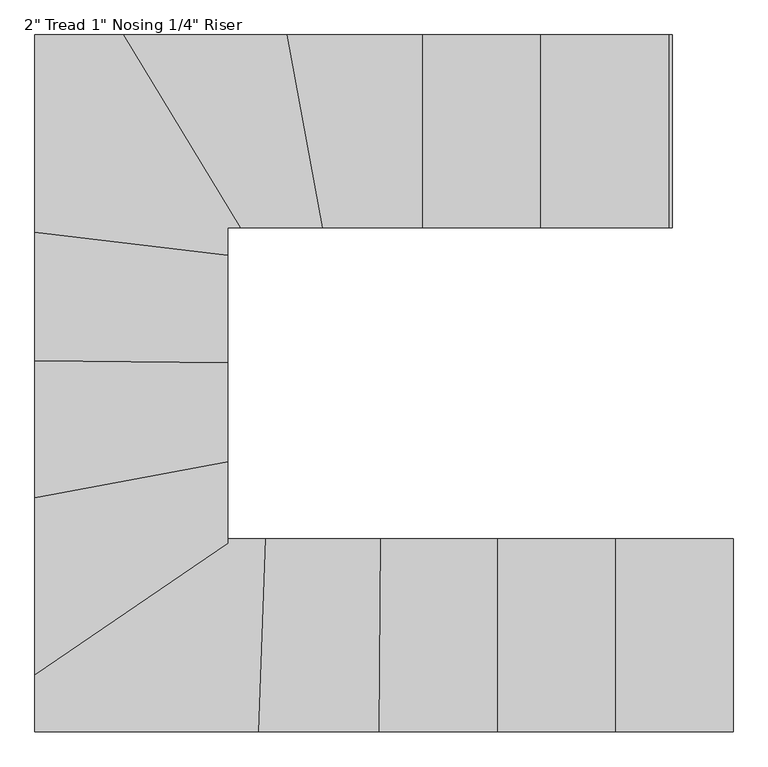
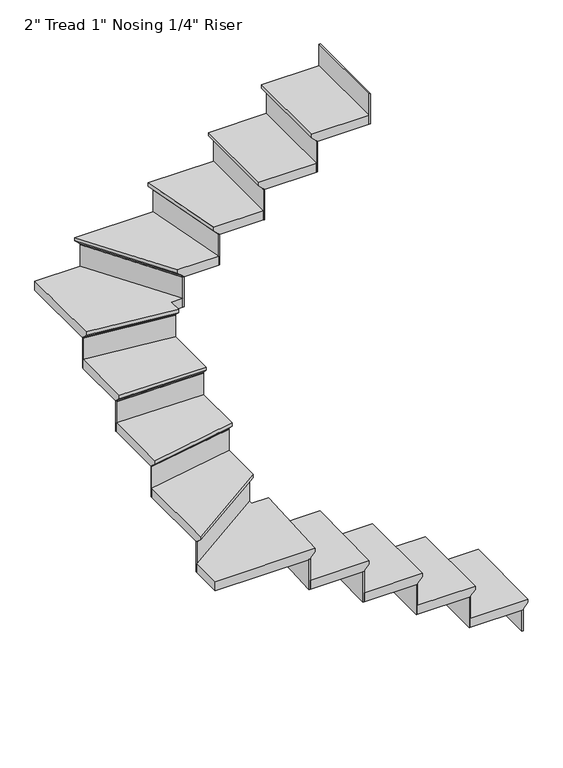
"""IFC4 building model written with IfcOpenShell, lengths in millimetres: stair flight geometry."""

from ifc_helpers import new_model, si_unit, origin, place, context, project, spatial, faceted_brep, source, transform, mapped, element, save


def stair_flight_132ddc74(model_context):
    return source(origin(), model_context, "Body", "Brep", [
        faceted_brep([(-10847.2047602, 4039.299435, 488.95), (-10847.2047602, 4039.299435, 508.0), (-10847.2047602, 3582.099435, 508.0), (-10847.2047602, 3582.099435, 488.95), (-10872.6047602, 4039.299435, 463.55), (-10872.6047602, 3582.099435, 463.55), (-11152.0047602, 4039.299435, 508.0), (-11152.0047602, 3582.099435, 508.0), (-10872.6047602, 3582.099435, 457.2), (-11152.0047602, 3582.099435, 457.2), (-11152.0047602, 4039.299435, 457.2), (-10872.6047602, 4039.299435, 457.2)], [[[0, 1, 2, 3]], [[4, 0, 3, 5]], [[2, 1, 6, 7]], [[8, 9, 10, 11]], [[2, 7, 9, 8, 5, 3]], [[8, 11, 4, 5]], [[6, 1, 0, 4, 11, 10]], [[7, 6, 10, 9]]]),
        faceted_brep([(-10872.6047602, 4039.299435, 457.2), (-10872.6047602, 4039.299435, 338.6666667), (-10878.9547602, 4039.299435, 338.6666667), (-10878.9547602, 4039.299435, 457.2), (-10872.6047602, 3582.099435, 457.2), (-10878.9547602, 3582.099435, 457.2), (-10878.9547602, 3582.099435, 338.6666667), (-10872.6047602, 3582.099435, 338.6666667)], [[[0, 1, 2, 3]], [[4, 5, 6, 7]], [[1, 0, 4, 7]], [[2, 1, 7, 6]], [[3, 2, 6, 5]], [[0, 3, 5, 4]]]),
        faceted_brep([(-11152.0047602, 4039.299435, 626.5333333), (-11152.0047602, 4039.299435, 457.2), (-11158.3547602, 4039.299435, 457.2), (-11158.3547602, 4039.299435, 626.5333333), (-11152.0047602, 3582.099435, 626.5333333), (-11158.3547602, 3582.099435, 626.5333333), (-11158.3547602, 3582.099435, 457.2), (-11152.0047602, 3582.099435, 457.2)], [[[0, 1, 2, 3]], [[4, 5, 6, 7]], [[1, 0, 4, 7]], [[2, 1, 7, 6]], [[3, 2, 6, 5]], [[0, 3, 5, 4]]]),
        faceted_brep([(-11126.6047602, 3582.099435, 677.3333333), (-11126.6047602, 4039.299435, 677.3333333), (-11431.4047602, 4039.299435, 677.3333333), (-11431.4047602, 3582.099435, 677.3333333), (-11152.0047602, 3582.099435, 626.5333333), (-11431.4047602, 3582.099435, 626.5333333), (-11431.4047602, 4039.299435, 626.5333333), (-11152.0047602, 4039.299435, 626.5333333), (-11152.0047602, 3582.099435, 632.8833333), (-11126.6047602, 3582.099435, 658.2833333), (-11152.0047602, 4039.299435, 632.8833333), (-11126.6047602, 4039.299435, 658.2833333)], [[[0, 1, 2, 3]], [[4, 5, 6, 7]], [[0, 3, 5, 4, 8, 9]], [[4, 7, 10, 8]], [[2, 1, 11, 10, 7, 6]], [[3, 2, 6, 5]], [[11, 1, 0, 9]], [[10, 11, 9, 8]]]),
        faceted_brep([(-11431.4047602, 4039.299435, 795.8666667), (-11431.4047602, 4039.299435, 626.5333333), (-11437.7547602, 4039.299435, 626.5333333), (-11437.7547602, 4039.299435, 795.8666667), (-11431.4047602, 3582.099435, 795.8666667), (-11437.7547602, 3582.099435, 795.8666667), (-11437.7547602, 3582.099435, 626.5333333), (-11431.4047602, 3582.099435, 626.5333333)], [[[0, 1, 2, 3]], [[4, 5, 6, 7]], [[1, 0, 4, 7]], [[2, 1, 7, 6]], [[3, 2, 6, 5]], [[0, 3, 5, 4]]]),
        faceted_brep([(-11406.0047602, 3582.099435, 846.6666667), (-11406.0047602, 4039.299435, 846.6666667), (-11708.6929844, 4039.299435, 846.6666667), (-11712.9187058, 3582.099435, 846.6666667), (-11431.4047602, 3582.099435, 795.8666667), (-11712.9187058, 3582.099435, 795.8666667), (-11708.6929844, 4039.299435, 795.8666667), (-11431.4047602, 4039.299435, 795.8666667), (-11431.4047602, 3582.099435, 802.2166667), (-11406.0047602, 3582.099435, 827.6166667), (-11431.4047602, 4039.299435, 802.2166667), (-11406.0047602, 4039.299435, 827.6166667)], [[[0, 1, 2, 3]], [[4, 5, 6, 7]], [[0, 3, 5, 4, 8, 9]], [[4, 7, 10, 8]], [[2, 1, 11, 10, 7, 6]], [[3, 2, 6, 5]], [[11, 1, 0, 9]], [[10, 11, 9, 8]]]),
        faceted_brep([(-11708.6929844, 4039.299435, 965.2), (-11708.6929844, 4039.299435, 795.8666667), (-11715.0432556, 4039.299435, 795.8666667), (-11715.0432556, 4039.299435, 965.2), (-11712.9187058, 3582.099435, 965.2), (-11719.268977, 3582.099435, 965.2), (-11719.268977, 3582.099435, 795.8666667), (-11712.9187058, 3582.099435, 795.8666667)], [[[0, 1, 2, 3]], [[4, 5, 6, 7]], [[1, 0, 4, 7]], [[2, 1, 7, 6]], [[3, 2, 6, 5]], [[0, 3, 5, 4]]]),
        faceted_brep([(-11687.5176209, 3582.099435, 1016.0), (-11683.2918995, 4039.299435, 1016.0), (-11981.9484639, 4039.299435, 1016.0), (-11998.4943115, 3582.099435, 1016.0), (-11712.9187058, 3582.099435, 965.2), (-11998.4943115, 3582.099435, 965.2), (-11981.9484639, 4039.299435, 965.2), (-11708.6929844, 4039.299435, 965.2), (-11712.9187058, 3582.099435, 971.55), (-11687.5176209, 3582.099435, 996.95), (-11708.6929844, 4039.299435, 971.55), (-11683.2918995, 4039.299435, 996.95)], [[[0, 1, 2, 3]], [[4, 5, 6, 7]], [[0, 3, 5, 4, 8, 9]], [[4, 7, 10, 8]], [[2, 1, 11, 10, 7, 6]], [[3, 2, 6, 5]], [[11, 1, 0, 9]], [[10, 11, 9, 8]]]),
        faceted_brep([(-11981.9484639, 4039.299435, 1134.5333333), (-11981.9484639, 4039.299435, 965.2), (-11988.3026208, 4039.299435, 965.2), (-11988.3026208, 4039.299435, 1134.5333333), (-11998.4943115, 3582.099435, 1134.5333333), (-12004.8484684, 3582.099435, 1134.5333333), (-12004.8484684, 3582.099435, 965.2), (-11998.4943115, 3582.099435, 965.2)], [[[0, 1, 2, 3]], [[4, 5, 6, 7]], [[1, 0, 4, 7]], [[2, 1, 7, 6]], [[3, 2, 6, 5]], [[0, 3, 5, 4]]]),
        faceted_brep([(-12501.9364521, 3747.8081502, 1185.3333333), (-12501.9364521, 3582.099435, 1185.3333333), (-11973.077684, 3582.099435, 1185.3333333), (-11956.5318364, 4039.299435, 1185.3333333), (-12044.7364521, 4039.299435, 1185.3333333), (-12044.7364521, 4058.9952275, 1185.3333333), (-12501.9364521, 3582.099435, 1134.5333333), (-12501.9364521, 3747.8081502, 1134.5333333), (-12044.7364521, 4058.9952275, 1134.5333333), (-12044.7364521, 4039.299435, 1134.5333333), (-11981.9484639, 4039.299435, 1134.5333333), (-11998.4943115, 3582.099435, 1134.5333333), (-11981.9484639, 4039.299435, 1140.8833333), (-11998.4943115, 3582.099435, 1140.8833333), (-11956.5318364, 4039.299435, 1166.2833333), (-11973.077684, 3582.099435, 1166.2833333)], [[[0, 1, 2, 3, 4, 5]], [[6, 7, 8, 9, 10, 11]], [[1, 0, 7, 6]], [[11, 10, 12, 13]], [[4, 3, 14, 12, 10, 9]], [[0, 5, 8, 7]], [[14, 3, 2, 15]], [[12, 14, 15, 13]], [[2, 1, 6, 11, 13, 15]], [[5, 4, 9, 8]]]),
        faceted_brep([(-12044.7364521, 4058.9952275, 1303.8666667), (-12044.7364521, 4058.9952275, 1134.5333333), (-12044.7364521, 4066.6765395, 1134.5333333), (-12044.7364521, 4066.6765395, 1303.8666667), (-12501.9364521, 3747.8081502, 1303.8666667), (-12501.9364521, 3755.4894621, 1303.8666667), (-12501.9364521, 3755.4894621, 1134.5333333), (-12501.9364521, 3747.8081502, 1134.5333333)], [[[0, 1, 2, 3]], [[4, 5, 6, 7]], [[1, 0, 4, 7]], [[2, 1, 7, 6]], [[3, 2, 6, 5]], [[0, 3, 5, 4]]]),
        faceted_brep([(-12501.9364521, 3717.0829023, 1354.6666667), (-12044.7364521, 4028.2699796, 1354.6666667), (-12044.7364521, 4246.917794, 1354.6666667), (-12501.9364521, 4162.7485719, 1354.6666667), (-12501.9364521, 3747.8081502, 1303.8666667), (-12501.9364521, 4162.7485719, 1303.8666667), (-12044.7364521, 4246.917794, 1303.8666667), (-12044.7364521, 4058.9952275, 1303.8666667), (-12501.9364521, 3747.8081502, 1310.2166667), (-12501.9364521, 3717.0829023, 1335.6166667), (-12044.7364521, 4058.9952275, 1310.2166667), (-12044.7364521, 4028.2699796, 1335.6166667)], [[[0, 1, 2, 3]], [[4, 5, 6, 7]], [[0, 3, 5, 4, 8, 9]], [[4, 7, 10, 8]], [[3, 2, 6, 5]], [[11, 1, 0, 9]], [[10, 11, 9, 8]], [[2, 1, 11, 10, 7, 6]]]),
        faceted_brep([(-12044.7364521, 4246.917794, 1473.2), (-12044.7364521, 4246.917794, 1303.8666667), (-12044.7364521, 4253.3745038, 1303.8666667), (-12044.7364521, 4253.3745038, 1473.2), (-12501.9364521, 4162.7485719, 1473.2), (-12501.9364521, 4169.2052817, 1473.2), (-12501.9364521, 4169.2052817, 1303.8666667), (-12501.9364521, 4162.7485719, 1303.8666667)], [[[0, 1, 2, 3]], [[4, 5, 6, 7]], [[1, 0, 4, 7]], [[2, 1, 7, 6]], [[3, 2, 6, 5]], [[0, 3, 5, 4]]]),
        faceted_brep([(-12501.9364521, 4136.921733, 1524.0), (-12044.7364521, 4221.0909551, 1524.0), (-12044.7364521, 4481.5064231, 1524.0), (-12501.9364521, 4486.1088388, 1524.0), (-12501.9364521, 4162.7485719, 1473.2), (-12501.9364521, 4486.1088388, 1473.2), (-12044.7364521, 4481.5064231, 1473.2), (-12044.7364521, 4246.917794, 1473.2), (-12501.9364521, 4162.7485719, 1479.55), (-12501.9364521, 4136.921733, 1504.95), (-12044.7364521, 4246.917794, 1479.55), (-12044.7364521, 4221.0909551, 1504.95)], [[[0, 1, 2, 3]], [[4, 5, 6, 7]], [[0, 3, 5, 4, 8, 9]], [[4, 7, 10, 8]], [[2, 1, 11, 10, 7, 6]], [[3, 2, 6, 5]], [[11, 1, 0, 9]], [[10, 11, 9, 8]]]),
        faceted_brep([(-12044.7364521, 4481.5064231, 1642.5333333), (-12044.7364521, 4481.5064231, 1473.2), (-12044.7364521, 4487.8567448, 1473.2), (-12044.7364521, 4487.8567448, 1642.5333333), (-12501.9364521, 4486.1088388, 1642.5333333), (-12501.9364521, 4492.4591605, 1642.5333333), (-12501.9364521, 4492.4591605, 1473.2), (-12501.9364521, 4486.1088388, 1473.2)], [[[0, 1, 2, 3]], [[4, 5, 6, 7]], [[1, 0, 4, 7]], [[2, 1, 7, 6]], [[3, 2, 6, 5]], [[0, 3, 5, 4]]]),
        faceted_brep([(-12501.9364521, 4460.7075518, 1693.3333333), (-12044.7364521, 4456.1051362, 1693.3333333), (-12044.7364521, 4736.0810551, 1693.3333333), (-12501.9364521, 4790.6927531, 1693.3333333), (-12501.9364521, 4486.1088388, 1642.5333333), (-12501.9364521, 4790.6927531, 1642.5333333), (-12044.7364521, 4736.0810551, 1642.5333333), (-12044.7364521, 4481.5064231, 1642.5333333), (-12501.9364521, 4486.1088388, 1648.8833333), (-12501.9364521, 4460.7075518, 1674.2833333), (-12044.7364521, 4481.5064231, 1648.8833333), (-12044.7364521, 4456.1051362, 1674.2833333)], [[[0, 1, 2, 3]], [[4, 5, 6, 7]], [[0, 3, 5, 4, 8, 9]], [[4, 7, 10, 8]], [[3, 2, 6, 5]], [[11, 1, 0, 9]], [[10, 11, 9, 8]], [[2, 1, 11, 10, 7, 6]]]),
        faceted_brep([(-12044.7364521, 4736.0810551, 1811.8666667), (-12044.7364521, 4736.0810551, 1642.5333333), (-12044.7364521, 4742.4761952, 1642.5333333), (-12044.7364521, 4742.4761952, 1811.8666667), (-12501.9364521, 4790.6927531, 1811.8666667), (-12501.9364521, 4797.0878931, 1811.8666667), (-12501.9364521, 4797.0878931, 1642.5333333), (-12501.9364521, 4790.6927531, 1642.5333333)], [[[0, 1, 2, 3]], [[4, 5, 6, 7]], [[1, 0, 4, 7]], [[2, 1, 7, 6]], [[3, 2, 6, 5]], [[0, 3, 5, 4]]]),
        faceted_brep([(-12261.8071685, 5233.099435, 1862.6666667), (-12501.9364521, 5233.099435, 1862.6666667), (-12501.9364521, 4765.112193, 1862.6666667), (-12044.7364521, 4710.5004951, 1862.6666667), (-12044.7364521, 4775.899435, 1862.6666667), (-11984.9256637, 4775.899435, 1862.6666667), (-12501.9364521, 5233.099435, 1811.8666667), (-12261.8071685, 5233.099435, 1811.8666667), (-11984.9256637, 4775.899435, 1811.8666667), (-12044.7364521, 4775.899435, 1811.8666667), (-12044.7364521, 4736.0810551, 1811.8666667), (-12501.9364521, 4790.6927531, 1811.8666667), (-12044.7364521, 4736.0810551, 1818.2166667), (-12501.9364521, 4790.6927531, 1818.2166667), (-12044.7364521, 4710.5004951, 1843.6166667), (-12501.9364521, 4765.112193, 1843.6166667)], [[[0, 1, 2, 3, 4, 5]], [[6, 7, 8, 9, 10, 11]], [[1, 0, 7, 6]], [[11, 10, 12, 13]], [[4, 3, 14, 12, 10, 9]], [[0, 5, 8, 7]], [[14, 3, 2, 15]], [[12, 14, 15, 13]], [[2, 1, 6, 11, 13, 15]], [[5, 4, 9, 8]]]),
        faceted_brep([(-11984.9256637, 4775.899435, 1981.2), (-11984.9256637, 4775.899435, 1811.8666667), (-11977.5019881, 4775.899435, 1811.8666667), (-11977.5019881, 4775.899435, 1981.2), (-12261.8071685, 5233.099435, 1981.2), (-12254.383493, 5233.099435, 1981.2), (-12254.383493, 5233.099435, 1811.8666667), (-12261.8071685, 5233.099435, 1811.8666667)], [[[0, 1, 2, 3]], [[4, 5, 6, 7]], [[1, 0, 4, 7]], [[2, 1, 7, 6]], [[3, 2, 6, 5]], [[0, 3, 5, 4]]]),
        faceted_brep([(-12291.5018706, 5233.099435, 2032.0), (-12014.6203657, 4775.899435, 2032.0), (-11794.3409035, 4775.899435, 2032.0), (-11877.5314837, 5233.099435, 2032.0), (-12261.8071685, 5233.099435, 1981.2), (-11877.5314837, 5233.099435, 1981.2), (-11794.3409035, 4775.899435, 1981.2), (-11984.9256637, 4775.899435, 1981.2), (-12261.8071685, 5233.099435, 1987.55), (-12291.5018706, 5233.099435, 2012.95), (-11984.9256637, 4775.899435, 1987.55), (-12014.6203657, 4775.899435, 2012.95)], [[[0, 1, 2, 3]], [[4, 5, 6, 7]], [[0, 3, 5, 4, 8, 9]], [[4, 7, 10, 8]], [[2, 1, 11, 10, 7, 6]], [[3, 2, 6, 5]], [[11, 1, 0, 9]], [[10, 11, 9, 8]]]),
        faceted_brep([(-11794.3409035, 4775.899435, 2150.5333333), (-11794.3409035, 4775.899435, 1981.2), (-11787.8866408, 4775.899435, 1981.2), (-11787.8866408, 4775.899435, 2150.5333333), (-11877.5314837, 5233.099435, 2150.5333333), (-11871.0772211, 5233.099435, 2150.5333333), (-11871.0772211, 5233.099435, 1981.2), (-11877.5314837, 5233.099435, 1981.2)], [[[0, 1, 2, 3]], [[4, 5, 6, 7]], [[1, 0, 4, 7]], [[2, 1, 7, 6]], [[3, 2, 6, 5]], [[0, 3, 5, 4]]]),
        faceted_brep([(-11903.3485343, 5233.099435, 2201.3333333), (-11820.157954, 4775.899435, 2201.3333333), (-11556.9532442, 4775.899435, 2201.3333333), (-11556.9532442, 5233.099435, 2201.3333333), (-11877.5314837, 5233.099435, 2150.5333333), (-11556.9532442, 5233.099435, 2150.5333333), (-11556.9532442, 4775.899435, 2150.5333333), (-11794.3409035, 4775.899435, 2150.5333333), (-11877.5314837, 5233.099435, 2156.8833333), (-11903.3485343, 5233.099435, 2182.2833333), (-11794.3409035, 4775.899435, 2156.8833333), (-11820.157954, 4775.899435, 2182.2833333)], [[[0, 1, 2, 3]], [[4, 5, 6, 7]], [[0, 3, 5, 4, 8, 9]], [[4, 7, 10, 8]], [[2, 1, 11, 10, 7, 6]], [[3, 2, 6, 5]], [[11, 1, 0, 9]], [[10, 11, 9, 8]]]),
        faceted_brep([(-11556.9532442, 4775.899435, 2319.8666667), (-11556.9532442, 4775.899435, 2150.5333333), (-11550.6032442, 4775.899435, 2150.5333333), (-11550.6032442, 4775.899435, 2319.8666667), (-11556.9532442, 5233.099435, 2319.8666667), (-11550.6032442, 5233.099435, 2319.8666667), (-11550.6032442, 5233.099435, 2150.5333333), (-11556.9532442, 5233.099435, 2150.5333333)], [[[0, 1, 2, 3]], [[4, 5, 6, 7]], [[1, 0, 4, 7]], [[2, 1, 7, 6]], [[3, 2, 6, 5]], [[0, 3, 5, 4]]]),
        faceted_brep([(-11582.3532442, 5233.099435, 2370.6666667), (-11582.3532442, 4775.899435, 2370.6666667), (-11277.5532442, 4775.899435, 2370.6666667), (-11277.5532442, 5233.099435, 2370.6666667), (-11556.9532442, 5233.099435, 2319.8666667), (-11277.5532442, 5233.099435, 2319.8666667), (-11277.5532442, 4775.899435, 2319.8666667), (-11556.9532442, 4775.899435, 2319.8666667), (-11556.9532442, 5233.099435, 2326.2166667), (-11582.3532442, 5233.099435, 2351.6166667), (-11556.9532442, 4775.899435, 2326.2166667), (-11582.3532442, 4775.899435, 2351.6166667)], [[[0, 1, 2, 3]], [[4, 5, 6, 7]], [[0, 3, 5, 4, 8, 9]], [[4, 7, 10, 8]], [[2, 1, 11, 10, 7, 6]], [[3, 2, 6, 5]], [[11, 1, 0, 9]], [[10, 11, 9, 8]]]),
        faceted_brep([(-11277.5532442, 4775.899435, 2489.2), (-11277.5532442, 4775.899435, 2319.8666667), (-11271.2032442, 4775.899435, 2319.8666667), (-11271.2032442, 4775.899435, 2489.2), (-11277.5532442, 5233.099435, 2489.2), (-11271.2032442, 5233.099435, 2489.2), (-11271.2032442, 5233.099435, 2319.8666667), (-11277.5532442, 5233.099435, 2319.8666667)], [[[0, 1, 2, 3]], [[4, 5, 6, 7]], [[1, 0, 4, 7]], [[2, 1, 7, 6]], [[3, 2, 6, 5]], [[0, 3, 5, 4]]]),
        faceted_brep([(-10998.1532442, 4775.899435, 2658.5333333), (-10998.1532442, 4775.899435, 2489.2), (-10991.8032442, 4775.899435, 2489.2), (-10991.8032442, 4775.899435, 2658.5333333), (-10998.1532442, 5233.099435, 2658.5333333), (-10991.8032442, 5233.099435, 2658.5333333), (-10991.8032442, 5233.099435, 2489.2), (-10998.1532442, 5233.099435, 2489.2)], [[[0, 1, 2, 3]], [[4, 5, 6, 7]], [[1, 0, 4, 7]], [[2, 1, 7, 6]], [[3, 2, 6, 5]], [[0, 3, 5, 4]]]),
        faceted_brep([(-11302.9532442, 5233.099435, 2540.0), (-11302.9532442, 4775.899435, 2540.0), (-10998.1532442, 4775.899435, 2540.0), (-10998.1532442, 5233.099435, 2540.0), (-11277.5532442, 5233.099435, 2489.2), (-10998.1532442, 5233.099435, 2489.2), (-10998.1532442, 4775.899435, 2489.2), (-11277.5532442, 4775.899435, 2489.2), (-11277.5532442, 5233.099435, 2495.55), (-11302.9532442, 5233.099435, 2520.95), (-11277.5532442, 4775.899435, 2495.55), (-11302.9532442, 4775.899435, 2520.95)], [[[0, 1, 2, 3]], [[4, 5, 6, 7]], [[0, 3, 5, 4, 8, 9]], [[4, 7, 10, 8]], [[2, 1, 11, 10, 7, 6]], [[3, 2, 6, 5]], [[11, 1, 0, 9]], [[10, 11, 9, 8]]]),
    ])


if __name__ == "__main__":
    model = new_model("IFC4")
    model_context = context("Model", 3, world=origin())
    ifc_project = project(units=[si_unit("LENGTHUNIT", "METRE", prefix="MILLI")], contexts=[model_context])
    site = spatial("IfcSite", under=ifc_project)
    building = spatial("IfcBuilding", under=site)
    placement = place(None, origin())
    stair_flight_shape = stair_flight_132ddc74(model_context)
    element("IfcStairFlight", 1, ObjectType="2\" Tread 1\" Nosing 1/4\" Riser", at=placement, inside=building, context=model_context, shape_type="MappedRepresentation", body=[
        mapped(stair_flight_shape, transform((0.0, 0.0, 0.0), x_axis=(1.0, 0.0, 0.0), y_axis=(0.0, 1.0, 0.0), z_axis=(0.0, 0.0, 1.0))),
    ])
    save(model, "model.ifc")
